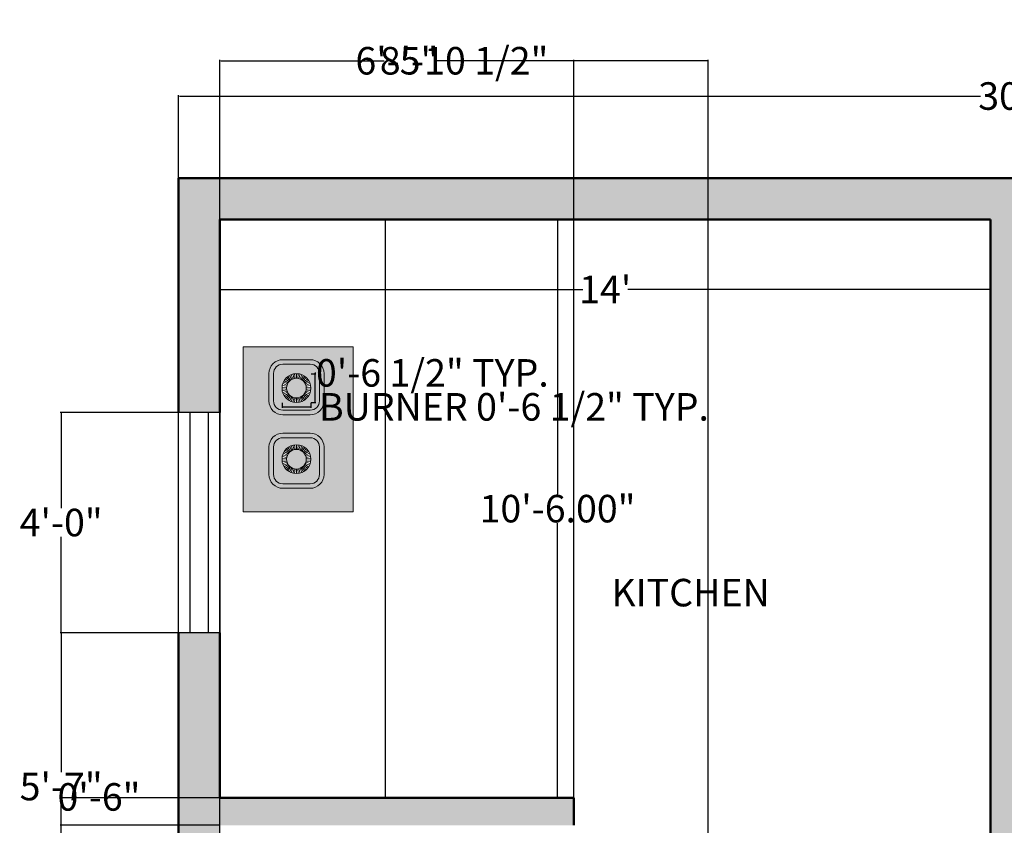
# Model space of a CAD drawing. Units: inches. Extents: x -19 to 426, y -15 to 535.
# Tile 3 of 4: x -12 to 202, y 359 to 535. Entities that reach past the tile are written whole.
import ezdxf

# ---------------------------------------------------------------- set-up
doc = ezdxf.new("R2010")
doc.units = ezdxf.units.IN
doc.header["$MEASUREMENT"] = 0
for name, color, linetype, lineweight in [('A-ANNO-DIMS', 3, 'Continuous', 18), ('A-AREA-IDEN', 7, 'Continuous', 25), ('A-EQPM', 8, 'Continuous', 18), ('A-EQPM-PATT', 9, 'Continuous', 13), ('A-FLOR-CABN', 40, 'Continuous', 25), ('A-GLAZ', 40, 'Continuous', 25), ('A-WALL', 7, 'Continuous', 50), ('A-WALL-PATT', 5, 'Continuous', 13)]:
    doc.layers.add(name, color=color, linetype=linetype, lineweight=lineweight)
doc.styles.get("Standard").update_dxf_attribs({"font": 'arial.ttf'})
doc.dimstyles.get("Standard").update_dxf_attribs({"dimtxt": 6, "dimasz": 0.18, "dimexe": 0.18, "dimexo": 0.0625, "dimgap": 0.09, "dimtad": 0, "dimtih": 1, "dimtoh": 1, "dimzin": 0, "dimdsep": 46, "dimlunit": 3, "dimtxsty": 'Standard', "dimcen": 0.09, "dimadec": 0, "dimazin": 0, "dimtfac": 1, "dimtofl": 0, "dimtmove": 0, "dimatfit": 3, "dimfxl": 1, "dimtolj": 1, "dimtzin": 0, "dimarcsym": 0})

# ---------------------------------------------------------------- blocks, each defined once
blk = doc.blocks.new('*D13')
at = {"layer": 'A-ANNO-DIMS', "color": 0, "lineweight": -2, "transparency": 16777216}
for p, q in [((31.43, 490.94), (31.43, 475.59)), ((199.43, 490.94), (199.43, 475.59)), ((31.61, 475.77), (110.53, 475.77)), ((199.25, 475.77), (120.33, 475.77))]:
    blk.add_line(p, q, dxfattribs=at)
at = {"layer": 'A-ANNO-DIMS', "color": 0, "transparency": 16777216}
for points in [[(31.61, 475.8), (31.61, 475.74), (31.43, 475.77)], [(199.25, 475.8), (199.25, 475.74), (199.43, 475.77)]]:
    blk.add_solid(points, dxfattribs=at)
at = {"layer": 'Defpoints', "color": 0, "transparency": 16777216}
for p in [(31.43, 491.01), (199.43, 491.01), (199.43, 475.77)]:
    blk.add_point(p, dxfattribs=at)
at = {"layer": 'A-ANNO-DIMS', "color": 0, "transparency": 16777216, "insert": (115.43, 475.77), "char_height": 6, "attachment_point": 5}
blk.add_mtext("\\A1;14'", dxfattribs=at)
blk = doc.blocks.new('*D14')
at = {"layer": 'A-ANNO-DIMS', "color": 0, "lineweight": -2, "transparency": 16777216}
for p, q in [((108.53, 491.01), (104.86, 491.01)), ((105.04, 490.83), (105.04, 431.16)), ((105.04, 365.19), (105.04, 424.85)), ((108.53, 365.01), (104.86, 365.01))]:
    blk.add_line(p, q, dxfattribs=at)
at = {"layer": 'A-ANNO-DIMS', "color": 0, "transparency": 16777216}
for points in [[(105.01, 490.83), (105.07, 490.83), (105.04, 491.01)], [(105.01, 365.19), (105.07, 365.19), (105.04, 365.01)]]:
    blk.add_solid(points, dxfattribs=at)
at = {"layer": 'Defpoints', "color": 0, "transparency": 16777216}
for p in [(105.04, 491.01), (108.59, 491.01), (108.59, 365.01)]:
    blk.add_point(p, dxfattribs=at)
at = {"layer": 'A-ANNO-DIMS', "color": 0, "transparency": 16777216, "insert": (105.04, 428.01), "char_height": 6, "attachment_point": 5}
blk.add_mtext('\\A1;10\'-6.00"', dxfattribs=at)
blk = doc.blocks.new('*D18')
at = {"layer": 'A-ANNO-DIMS', "color": 0, "lineweight": -2, "transparency": 16777216}
for p, q in [((22.43, 500.07), (22.43, 518.1)), ((22.61, 517.92), (197.25, 517.92)), ((382.25, 517.92), (207.61, 517.92)), ((382.43, 500.07), (382.43, 518.1))]:
    blk.add_line(p, q, dxfattribs=at)
at = {"layer": 'A-ANNO-DIMS', "color": 0, "transparency": 16777216}
for points in [[(22.61, 517.95), (22.61, 517.89), (22.43, 517.92)], [(382.25, 517.95), (382.25, 517.89), (382.43, 517.92)]]:
    blk.add_solid(points, dxfattribs=at)
at = {"layer": 'Defpoints', "color": 0, "transparency": 16777216}
for p in [(382.43, 517.92), (22.43, 500.01), (382.43, 500.01)]:
    blk.add_point(p, dxfattribs=at)
at = {"layer": 'A-ANNO-DIMS', "color": 0, "transparency": 16777216, "insert": (202.43, 517.92), "char_height": 6, "attachment_point": 5}
blk.add_mtext("\\A1;30'", dxfattribs=at)
blk = doc.blocks.new('COOKTOP-BURNER')
for p, q in [((1.2, 4.05), (0.3, 4.48)), ((1.33, 4.29), (0.49, 4.82)), ((1.49, 4.5), (0.72, 5.14)), ((1.68, 4.7), (0.99, 5.43)), ((1.88, 4.87), (1.29, 5.68)), ((2.11, 5.02), (1.63, 5.89)), ((2.35, 5.13), (1.98, 6.06)), ((2.61, 5.21), (2.36, 6.18)), ((2.87, 5.26), (2.75, 6.26)), ((3.14, 5.28), (3.14, 6.28)), ((3.41, 5.26), (3.53, 6.26)), ((3.67, 5.21), (3.92, 6.18)), ((3.93, 5.13), (4.3, 6.06)), ((4.17, 5.02), (4.65, 5.89)), ((4.4, 4.87), (4.99, 5.68)), ((4.61, 4.7), (5.29, 5.43)), ((4.79, 4.5), (5.56, 5.14)), ((4.95, 4.29), (5.79, 4.82)), ((5.08, 4.05), (5.98, 4.48)), ((1, 3.27), (0.01, 3.34)), ((1, 3.01), (0.01, 2.94)), ((1.04, 3.54), (0.06, 3.73)), ((1.04, 2.74), (0.06, 2.55)), ((1.1, 3.8), (0.15, 4.11)), ((1.1, 2.48), (0.15, 2.17)), ((1.2, 2.23), (0.3, 1.8)), ((5.08, 2.23), (5.98, 1.8)), ((5.18, 3.8), (6.13, 4.11)), ((5.18, 2.48), (6.13, 2.17)), ((5.24, 3.54), (6.22, 3.73)), ((5.24, 2.74), (6.22, 2.55)), ((5.28, 3.27), (6.27, 3.34)), ((5.28, 3.01), (6.27, 2.94)), ((1.33, 1.99), (0.49, 1.46)), ((1.49, 1.78), (0.72, 1.14)), ((1.68, 1.58), (0.99, 0.85)), ((1.88, 1.41), (1.29, 0.6)), ((2.11, 1.26), (1.63, 0.39)), ((2.35, 1.15), (1.98, 0.22)), ((2.61, 1.07), (2.36, 0.1)), ((2.87, 1.02), (2.75, 0.02)), ((3.14, 1), (3.14, 0)), ((3.41, 1.02), (3.53, 0.02)), ((3.67, 1.07), (3.92, 0.1)), ((3.93, 1.15), (4.3, 0.22)), ((4.17, 1.26), (4.65, 0.39)), ((4.4, 1.41), (4.99, 0.6)), ((4.61, 1.58), (5.29, 0.85)), ((4.79, 1.78), (5.56, 1.14)), ((4.95, 1.99), (5.79, 1.46))]:
    blk.add_line(p, q)
for radius in [3.14, 2.14, 2.14, 2.14, 2.14, 2.14, 2.14, 2.14, 2.14, 2.14, 2.14, 2.14, 2.14, 2.14, 2.14, 2.14, 2.14, 2.14, 2.14, 2.14, 2.14, 2.14, 2.14, 2.14, 2.14, 2.14, 2.14, 2.14, 2.14, 2.14, 2.14, 2.14, 2.14, 2.14, 2.14, 2.14, 2.14, 2.14, 2.14, 2.14, 2.14, 2.14, 2.14, 2.14, 2.14, 2.14, 2.14, 2.14, 2.14, 2.14, 2.14]:
    blk.add_circle((3.14, 3.14), radius)
blk = doc.blocks.new('*D28')
at = {"layer": 'A-ANNO-DIMS', "color": 0, "lineweight": -2, "transparency": 16777216}
for p, q in [((44.98, 451.07), (44.98, 450.01)), ((51.26, 451.07), (51.26, 450.01)), ((45.16, 450.19), (51.08, 450.19)), ((51.26, 450.19), (51.44, 450.19))]:
    blk.add_line(p, q, dxfattribs=at)
at = {"layer": 'A-ANNO-DIMS', "color": 0, "transparency": 16777216}
for points in [[(45.16, 450.22), (45.16, 450.16), (44.98, 450.19)], [(51.08, 450.22), (51.08, 450.16), (51.26, 450.19)]]:
    blk.add_solid(points, dxfattribs=at)
at = {"layer": 'Defpoints', "color": 0, "transparency": 16777216}
for p in [(44.98, 451.13), (51.26, 451.13), (51.26, 450.19)]:
    blk.add_point(p, dxfattribs=at)
at = {"layer": 'A-ANNO-DIMS', "color": 0, "transparency": 16777216, "insert": (95.54, 450.19), "char_height": 6, "attachment_point": 5}
blk.add_mtext('\\A1;BURNER 0\'-6 1/2" TYP.', dxfattribs=at)
blk = doc.blocks.new('*D29')
at = {"layer": 'A-ANNO-DIMS', "color": 0, "lineweight": -2, "transparency": 16777216}
for p, q in [((51.32, 457.41), (52.38, 457.41)), ((52.2, 457.41), (52.2, 457.59)), ((52.2, 457.59), (52.38, 457.59)), ((52.2, 451.31), (52.2, 457.23)), ((51.32, 451.13), (52.38, 451.13))]:
    blk.add_line(p, q, dxfattribs=at)
at = {"layer": 'A-ANNO-DIMS', "color": 0, "transparency": 16777216}
for points in [[(52.17, 457.23), (52.23, 457.23), (52.2, 457.41)], [(52.17, 451.31), (52.23, 451.31), (52.2, 451.13)]]:
    blk.add_solid(points, dxfattribs=at)
at = {"layer": 'Defpoints', "color": 0, "transparency": 16777216}
for p in [(51.26, 457.41), (52.2, 457.41), (51.26, 451.13)]:
    blk.add_point(p, dxfattribs=at)
at = {"layer": 'A-ANNO-DIMS', "color": 0, "transparency": 16777216, "insert": (77.75, 457.59), "char_height": 6, "attachment_point": 5}
blk.add_mtext('\\A1;0\'-6 1/2" TYP.', dxfattribs=at)
blk = doc.blocks.new('*D41')
at = {"layer": 'A-ANNO-DIMS', "color": 0, "lineweight": -2, "transparency": 16777216}
for p, q in [((22.37, 400.98), (-3.35, 400.98)), ((-3.17, 400.8), (-3.17, 370.59)), ((-3.17, 334.1), (-3.17, 364.31)), ((22.37, 333.92), (-3.35, 333.92))]:
    blk.add_line(p, q, dxfattribs=at)
at = {"layer": 'A-ANNO-DIMS', "color": 0, "transparency": 16777216}
for points in [[(-3.2, 400.8), (-3.14, 400.8), (-3.17, 400.98)], [(-3.2, 334.1), (-3.14, 334.1), (-3.17, 333.92)]]:
    blk.add_solid(points, dxfattribs=at)
at = {"layer": 'Defpoints', "color": 0, "transparency": 16777216}
for p in [(-3.17, 400.98), (22.43, 400.98), (22.43, 333.92)]:
    blk.add_point(p, dxfattribs=at)
at = {"layer": 'A-ANNO-DIMS', "color": 0, "transparency": 16777216, "insert": (-3.17, 367.45), "char_height": 6, "attachment_point": 5}
blk.add_mtext('\\A1;5\'-7"', dxfattribs=at)
blk = doc.blocks.new('*D42')
at = {"layer": 'A-ANNO-DIMS', "color": 0, "lineweight": -2, "transparency": 16777216}
for p, q in [((22.37, 448.98), (-3.35, 448.98)), ((-3.17, 448.8), (-3.17, 428.13)), ((-3.17, 401.16), (-3.17, 421.83)), ((22.37, 400.98), (-3.35, 400.98))]:
    blk.add_line(p, q, dxfattribs=at)
at = {"layer": 'A-ANNO-DIMS', "color": 0, "transparency": 16777216}
for points in [[(-3.2, 448.8), (-3.14, 448.8), (-3.17, 448.98)], [(-3.2, 401.16), (-3.14, 401.16), (-3.17, 400.98)]]:
    blk.add_solid(points, dxfattribs=at)
at = {"layer": 'Defpoints', "color": 0, "transparency": 16777216}
for p in [(-3.17, 448.98), (22.43, 448.98), (22.43, 400.98)]:
    blk.add_point(p, dxfattribs=at)
at = {"layer": 'A-ANNO-DIMS', "color": 0, "transparency": 16777216, "insert": (-3.17, 424.98), "char_height": 6, "attachment_point": 5}
blk.add_mtext('\\A1;4\'-0"', dxfattribs=at)
blk = doc.blocks.new('*D51')
at = {"layer": 'A-ANNO-DIMS', "color": 0, "lineweight": -2, "transparency": 16777216}
for p, q in [((31.43, 365.07), (31.43, 525.79)), ((31.61, 525.61), (61.93, 525.61)), ((108.41, 525.61), (78.09, 525.61)), ((108.59, 365.07), (108.59, 525.79))]:
    blk.add_line(p, q, dxfattribs=at)
at = {"layer": 'A-ANNO-DIMS', "color": 0, "transparency": 16777216}
for points in [[(31.61, 525.64), (31.61, 525.58), (31.43, 525.61)], [(108.41, 525.64), (108.41, 525.58), (108.59, 525.61)]]:
    blk.add_solid(points, dxfattribs=at)
at = {"layer": 'Defpoints', "color": 0, "transparency": 16777216}
for p in [(108.59, 525.61), (31.43, 365.01), (108.59, 365.01)]:
    blk.add_point(p, dxfattribs=at)
at = {"layer": 'A-ANNO-DIMS', "color": 0, "transparency": 16777216, "insert": (70.01, 525.61), "char_height": 6, "attachment_point": 5}
blk.add_mtext('\\A1;6\'-5"', dxfattribs=at)
blk = doc.blocks.new('*D52')
at = {"layer": 'A-ANNO-DIMS', "color": 0, "lineweight": -2, "transparency": 16777216}
for p, q in [((31.43, 239.07), (31.43, 525.79)), ((31.61, 525.61), (67.28, 525.61)), ((137.72, 525.61), (102.06, 525.61)), ((137.9, 239.07), (137.9, 525.79))]:
    blk.add_line(p, q, dxfattribs=at)
at = {"layer": 'A-ANNO-DIMS', "color": 0, "transparency": 16777216}
for points in [[(31.61, 525.64), (31.61, 525.58), (31.43, 525.61)], [(137.72, 525.64), (137.72, 525.58), (137.9, 525.61)]]:
    blk.add_solid(points, dxfattribs=at)
at = {"layer": 'Defpoints', "color": 0, "transparency": 16777216}
for p in [(137.9, 525.61), (31.43, 239.01), (137.9, 239.01)]:
    blk.add_point(p, dxfattribs=at)
at = {"layer": 'A-ANNO-DIMS', "color": 0, "transparency": 16777216, "insert": (84.67, 525.61), "char_height": 6, "attachment_point": 5}
blk.add_mtext('\\A1;8\'-10 1/2"', dxfattribs=at)
blk = doc.blocks.new('*D59')
at = {"layer": 'A-ANNO-DIMS', "color": 0, "lineweight": -2, "transparency": 16777216}
for p, q in [((31.37, 365.01), (-3.35, 365.01)), ((-3.17, 365.01), (-3.17, 365.19)), ((-3.17, 365.19), (-2.99, 365.19)), ((-3.17, 359.19), (-3.17, 364.83)), ((31.37, 359.01), (-3.35, 359.01))]:
    blk.add_line(p, q, dxfattribs=at)
at = {"layer": 'A-ANNO-DIMS', "color": 0, "transparency": 16777216}
for points in [[(-3.2, 364.83), (-3.14, 364.83), (-3.17, 365.01)], [(-3.2, 359.19), (-3.14, 359.19), (-3.17, 359.01)]]:
    blk.add_solid(points, dxfattribs=at)
at = {"layer": 'Defpoints', "color": 0, "transparency": 16777216}
for p in [(-3.17, 365.01), (31.43, 365.01), (31.43, 359.01)]:
    blk.add_point(p, dxfattribs=at)
at = {"layer": 'A-ANNO-DIMS', "color": 0, "transparency": 16777216, "insert": (5.08, 365.19), "char_height": 6, "attachment_point": 5}
blk.add_mtext('\\A1;0\'-6"', dxfattribs=at)

msp = doc.modelspace()

# ---------------------------------------------------------------- hatches: boundary and pattern name
at = {"layer": 'A-EQPM-PATT'}
h = msp.add_hatch(color=256, dxfattribs=at)
h.dxf.hatch_style = 1
h.paths.add_polyline_path([(60.504, 463.304), (36.504, 463.304), (36.504, 427.304), (60.504, 427.304)])
h.paths.add_polyline_path([(42.132, 451.47), (42.132, 457.47, -0.4142136), (45.132, 460.47), (51.132, 460.47, -0.4142136), (54.132, 457.47), (54.132, 451.47, -0.4142136), (51.132, 448.47), (45.132, 448.47, -0.4142136)], flags=16)
h.paths.add_polyline_path([(44.981, 454.274, -1), (51.261, 454.274, -1)], flags=0)
h.paths.add_polyline_path([(45.981, 454.274, -1), (50.261, 454.274, -1)], flags=0)
h.paths.add_polyline_path([(45.132, 444.442), (51.132, 444.442, -0.4142136), (54.132, 441.442), (54.132, 435.442, -0.4142136), (51.132, 432.442), (45.132, 432.442, -0.4142136), (42.132, 435.442), (42.132, 441.442, -0.4142136)], flags=16)
h.paths.add_polyline_path([(51.261, 438.787, -1), (44.981, 438.787, -1)], flags=0)
h.paths.add_polyline_path([(50.261, 438.787, -1), (45.981, 438.787, -1)], flags=0)
h = msp.add_hatch(color=256, dxfattribs=at)
h.dxf.hatch_style = 1
h.paths.add_polyline_path([(54.132, 441.442, 0.4142136), (51.132, 444.442), (45.132, 444.442, 0.4142136), (42.132, 441.442), (42.132, 435.442, 0.4142136), (45.132, 432.442), (51.132, 432.442, 0.4142136), (54.132, 435.442)])
h.paths.add_polyline_path([(43.132, 441.442, -0.4142136), (45.132, 443.442), (51.132, 443.442, -0.4142136), (53.132, 441.442), (53.132, 435.442, -0.4142136), (51.132, 433.442), (45.132, 433.442, -0.4142136), (43.132, 435.442)], flags=16)
h.paths.add_polyline_path([(44.981, 438.787, -1), (51.261, 438.787, -1)], flags=0)
h.paths.add_polyline_path([(45.981, 438.787, -1), (50.261, 438.787, -1)], flags=0)
h.paths.add_polyline_path([(54.132, 457.47, 0.4142136), (51.132, 460.47), (45.132, 460.47, 0.4142136), (42.132, 457.47), (42.132, 451.47, 0.4142136), (45.132, 448.47), (51.132, 448.47, 0.4142136), (54.132, 451.47)])
h.paths.add_polyline_path([(43.132, 457.47, -0.4142136), (45.132, 459.47), (51.132, 459.47, -0.4142136), (53.132, 457.47), (53.132, 451.47, -0.4142136), (51.132, 449.47), (45.132, 449.47, -0.4142136), (43.132, 451.47)], flags=16)
h.paths.add_polyline_path([(51.261, 454.274, -1), (44.981, 454.274, -1)], flags=0)
h.paths.add_polyline_path([(50.261, 454.274, -1), (45.981, 454.274, -1)], flags=0)
h = msp.add_hatch(color=256, dxfattribs=at)
h.dxf.hatch_style = 1
h.paths.add_polyline_path([(53.132, 457.47, 0.4142136), (51.132, 459.47), (45.132, 459.47, 0.4142136), (43.132, 457.47), (43.132, 451.47, 0.4142136), (45.132, 449.47), (51.132, 449.47, 0.4142136), (53.132, 451.47)])
h.paths.add_polyline_path([(51.261, 454.274, -1), (44.981, 454.274, -1)], flags=16)
h.paths.add_polyline_path([(50.261, 454.274, -1), (45.981, 454.274, -1)], flags=0)
h.paths.add_polyline_path([(51.132, 443.442), (45.132, 443.442, 0.4142136), (43.132, 441.442), (43.132, 435.442, 0.4142136), (45.132, 433.442), (51.132, 433.442, 0.4142136), (53.132, 435.442), (53.132, 441.442, 0.4142136)])
h.paths.add_polyline_path([(51.261, 438.787, -1), (44.981, 438.787, -1)], flags=16)
h.paths.add_polyline_path([(50.261, 438.787, -1), (45.981, 438.787, -1)], flags=0)
h = msp.add_hatch(color=256, dxfattribs=at)
h.dxf.hatch_style = 1
h.paths.add_polyline_path([(45.981, 454.274, 1), (50.261, 454.274, 1)])
h.paths.add_polyline_path([(50.261, 438.787, 1), (45.981, 438.787, 1)])
at = {"layer": 'A-WALL-PATT'}
h = msp.add_hatch(color=256, dxfattribs=at)
h.dxf.hatch_style = 1
h.paths.add_polyline_path([(205.432, 491.007), (254.275, 491.007), (254.275, 500.007), (22.432, 500.007), (22.432, 449.048), (31.432, 449.048), (31.432, 491.007), (199.432, 491.007), (199.432, 312.007), (225.033, 312.007), (225.033, 315.882), (225.033, 317.007), (205.432, 317.007)])
h.paths.add_polyline_path([(382.432, 500.007), (314.275, 500.007), (314.275, 491.007), (373.432, 491.007), (373.432, 423.411), (382.432, 423.411)])
h.paths.add_polyline_path([(382.432, 363.411), (373.432, 363.411), (373.432, 317.007), (250.847, 317.007, -0.0108825), (250.871, 315.882), (250.871, 312.007), (296.432, 312.007), (296.432, 262.945), (299.196, 262.945, -0.0304399), (301.432, 262.809), (301.432, 312.007), (373.432, 312.007), (373.432, 284.151), (382.432, 284.151)])
h = msp.add_hatch(color=256, dxfattribs=at)
h.dxf.hatch_style = 1
h.paths.add_polyline_path([(108.594, 365.007), (31.432, 365.007), (31.432, 400.979), (22.432, 400.979), (22.432, 333.921), (31.432, 333.921), (31.432, 359.007), (108.594, 359.007)])

# ---------------------------------------------------------------- linework, layer by layer
at = {"layer": 'A-EQPM'}
msp.add_line((36.504, 427.304), (60.504, 427.304), dxfattribs=at)
msp.add_lwpolyline([(36.504, 427.304), (36.504, 463.304), (60.504, 463.304), (60.504, 427.304)], dxfattribs=at)
msp.add_lwpolyline([(45.132, 448.47, -0.4142136), (42.132, 451.47), (42.132, 457.47, -0.4142136), (45.132, 460.47), (51.132, 460.47, -0.4142136), (54.132, 457.47), (54.132, 451.47, -0.4142136), (51.132, 448.47), (45.132, 448.47)], format="xyb", dxfattribs=at)
for points in [[(45.132, 449.47, -0.4142136), (43.132, 451.47), (43.132, 457.47, -0.4142136), (45.132, 459.47), (51.132, 459.47, -0.4142136), (53.132, 457.47), (53.132, 451.47, -0.4142136), (51.132, 449.47)], [(51.132, 432.442), (45.132, 432.442, -0.4142136), (42.132, 435.442), (42.132, 441.442, -0.4142136), (45.132, 444.442), (51.132, 444.442, -0.4142136), (54.132, 441.442), (54.132, 435.442, -0.4142136)], [(51.132, 433.442), (45.132, 433.442, -0.4142136), (43.132, 435.442), (43.132, 441.442, -0.4142136), (45.132, 443.442), (51.132, 443.442, -0.4142136), (53.132, 441.442), (53.132, 435.442, -0.4142136)]]:
    msp.add_lwpolyline(points, format="xyb", close=True, dxfattribs=at)
at = {"layer": 'A-FLOR-CABN'}
for points in [[(67.432, 491.007), (67.432, 448.979)], [(67.432, 491.007), (67.432, 365.007)]]:
    msp.add_lwpolyline(points, dxfattribs=at)
at = {"layer": 'A-GLAZ'}
for p, q in [((24.932, 400.979), (24.932, 449.048)), ((28.932, 400.979), (28.932, 449.048))]:
    msp.add_line(p, q, dxfattribs=at)
msp.add_lwpolyline([(22.432, 449.048), (31.432, 449.048), (31.432, 400.979), (22.432, 400.979)], close=True, dxfattribs=at)
at = {"layer": 'A-WALL'}
msp.add_line((108.594, 365.007), (108.594, 359.007), dxfattribs=at)
for points in [[(254.275, 500.007), (22.432, 500.007), (22.432, 448.979)], [(31.432, 491.007), (31.432, 448.979)], [(199.432, 491.007), (31.432, 491.007)], [(199.432, 491.007), (199.432, 312.007)], [(22.432, 400.979), (22.432, 333.874)], [(31.432, 400.979), (31.432, 365.007)], [(108.594, 365.007), (31.432, 365.007)]]:
    msp.add_lwpolyline(points, dxfattribs=at)

# ---------------------------------------------------------------- block references
at = {"layer": 'A-EQPM'}
for p in [(44.981, 451.133), (44.981, 435.647)]:
    msp.add_blockref('COOKTOP-BURNER', p, dxfattribs=at)

# ---------------------------------------------------------------- texts
at = {"layer": 'A-AREA-IDEN', "insert": (116.782, 412.709), "char_height": 6, "attachment_point": 1}
msp.add_mtext_dynamic_manual_height_columns('{KITCHEN }', width=105.43776, gutter_width=1, heights=[0.207], dxfattribs=at)

# ---------------------------------------------------------------- dimensions: what is measured, and where the dimension line sits
at = {"layer": 'A-ANNO-DIMS'}
for base, p1, p2, override, picture, middle in [((137.904, 525.607), (31.432, 239.007), (137.904, 239.007), {"dimdec": 1, "dimlfac": 1, "dimrnd": 0, "dimzin": 1, "dimdsep": 46, "dimlunit": 4, "dimfrac": 2}, '*D52', (84.668, 525.607)), ((108.594, 525.607), (31.432, 365.007), (108.594, 365.007), {"dimdec": 1, "dimlfac": 1, "dimrnd": 0, "dimzin": 1, "dimdsep": 46, "dimlunit": 4, "dimfrac": 2}, '*D51', (70.013, 525.607)), ((382.432, 517.915), (22.432, 500.007), (382.432, 500.007), {"dimclrd": 0, "dimclre": 0, "dimclrt": 0}, '*D18', (202.432, 517.915)), ((199.432, 475.771), (31.432, 491.007), (199.432, 491.007), {"dimclrd": 0, "dimclre": 0, "dimclrt": 0}, '*D13', (115.432, 475.771))]:
    dim = msp.add_linear_dim(base=base, p1=p1, p2=p2, dimstyle='Standard', override=override, dxfattribs=at)
    dim.commit()
    dim.dimension.update_dxf_attribs({"geometry": picture, "text_midpoint": middle})
for base, p1, p2, override, picture, middle in [((105.044, 491.007), (108.594, 365.007), (108.594, 491.007), {"dimclrd": 0, "dimclre": 0, "dimclrt": 0}, '*D14', (105.044, 428.007)), ((-3.168, 448.979), (22.432, 400.979), (22.432, 448.979), {"dimdec": 1, "dimlfac": 1, "dimrnd": 0, "dimzin": 1, "dimdsep": 46, "dimlunit": 4, "dimfrac": 2}, '*D42', (-3.168, 424.979)), ((-3.168, 400.979), (22.432, 333.921), (22.432, 400.979), {"dimdec": 1, "dimlfac": 1, "dimrnd": 0, "dimzin": 1, "dimdsep": 46, "dimlunit": 4, "dimfrac": 2}, '*D41', (-3.168, 367.45)), ((-3.168, 365.007), (31.432, 359.007), (31.432, 365.007), {"dimdec": 1, "dimlfac": 1, "dimrnd": 0, "dimzin": 1, "dimdsep": 46, "dimlunit": 4, "dimfrac": 2}, '*D59', (5.077, 365.187))]:
    dim = msp.add_linear_dim(base=base, p1=p1, p2=p2, angle=90, dimstyle='Standard', override=override, dxfattribs=at)
    dim.commit()
    dim.dimension.update_dxf_attribs({"geometry": picture, "text_midpoint": middle})
dim = msp.add_linear_dim(base=(52.203, 457.414), p1=(51.261, 451.133), p2=(51.261, 457.414), angle=90, text='<> TYP.', dimstyle='Standard', override={"dimdec": 1, "dimlfac": 1, "dimrnd": 0, "dimzin": 1, "dimdsep": 46, "dimlunit": 4, "dimfrac": 2}, dxfattribs=at)
dim.commit()
dim.dimension.update_dxf_attribs({"geometry": '*D29', "text_midpoint": (77.75, 457.594)})
dim = msp.add_linear_dim(base=(51.261, 450.191), p1=(44.981, 451.133), p2=(51.261, 451.133), text='BURNER <> TYP.', dimstyle='Standard', override={"dimdec": 1, "dimlfac": 1, "dimrnd": 0, "dimzin": 1, "dimdsep": 46, "dimlunit": 4, "dimfrac": 2}, dxfattribs=at)
dim.commit()
dim.dimension.update_dxf_attribs({"geometry": '*D28', "text_midpoint": (95.537, 450.191)})

doc.saveas('drawing.dxf')
